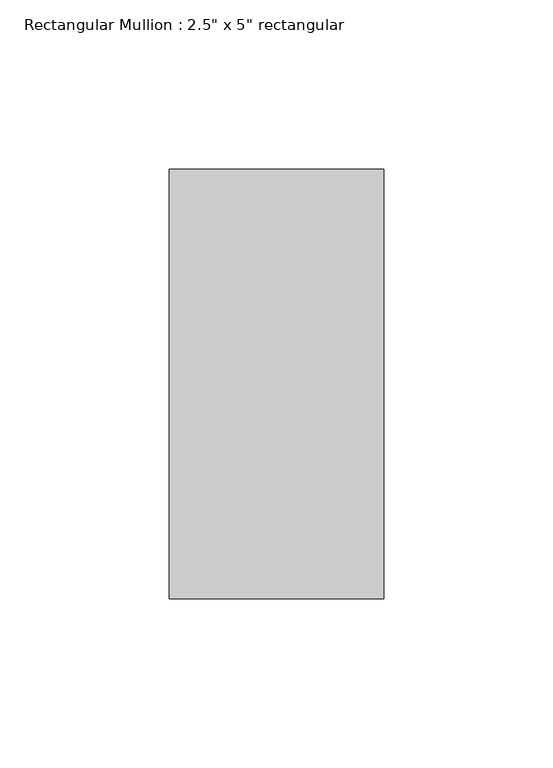
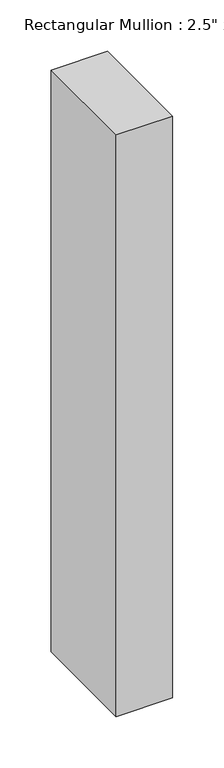
"""IFC4 building model written with IfcOpenShell, lengths in millimetres: member geometry."""

from ifc_helpers import new_model, si_unit, frame, origin, place, context, project, spatial, polyline, outline, extrude, source, transform, mapped, element, save


def member_5f1d7e17(model_context):
    return source(origin(), model_context, "Body", "SweptSolid", [
        extrude(outline(polyline([(0.0, 63.5), (0.0, -63.5), (-63.5, -63.5), (-63.5, 63.5), (0.0, 63.5)])), frame((0.0, 0.0, -692.15), z_axis=(0.0, 0.0, 1.0), x_axis=(1.0, 0.0, 0.0)), (0.0, 0.0, 1.0), 692.15),
    ])


if __name__ == "__main__":
    model = new_model("IFC4")
    model_context = context("Model", 3, world=origin())
    ifc_project = project(units=[si_unit("LENGTHUNIT", "METRE", prefix="MILLI")], contexts=[model_context])
    site = spatial("IfcSite", under=ifc_project)
    building = spatial("IfcBuilding", under=site)
    placement = place(None, origin())
    member_shape = member_5f1d7e17(model_context)
    element("IfcMember", 1, ObjectType="Rectangular Mullion : 2.5\" x 5\" rectangular", at=placement, inside=building, context=model_context, shape_type="MappedRepresentation", body=[
        mapped(member_shape, transform((0.0, 0.0, 0.0), x_axis=(1.0, 0.0, 0.0), y_axis=(0.0, 1.0, 0.0), z_axis=(0.0, 0.0, 1.0))),
    ])
    save(model, "model.ifc")

# Revit data of these elements
# Type "Rectangular Mullion : 2.5\" x 5\" rectangular"
#   built-in parameter 1007304 = 0.416667 (stored number, unit not read)
#   built-in parameter 1007301 = 0.104167 (stored number, unit not read)
#   built-in parameter 1007300 = 0.104167 (stored number, unit not read)
# Element 1 (IfcMember, "Rectangular Mullion : 2.5\" x 5\" rectangular")
#   Materials on its faces: "Aluminum"
# Materials
#   "Aluminum": class "Metal", colour RGB 247 247 247, transparency 0, Description = "Aluminum 6061", Cost = 0
